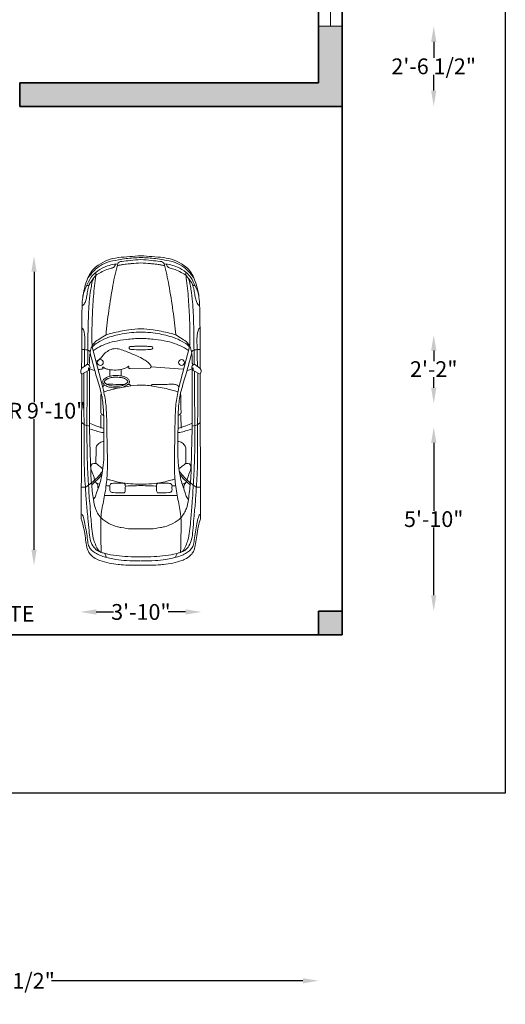
# Model space of a CAD drawing. Units: inches. Extents: x 1054 to 1577, y 4847 to 5610.
# Tile 2 of 5: x 1393 to 1577, y 4847 to 5221. Entities that reach past the tile are written whole.
import ezdxf

# ---------------------------------------------------------------- set-up
doc = ezdxf.new("R2010")
doc.units = ezdxf.units.IN
doc.header["$MEASUREMENT"] = 0
for name, color, linetype, lineweight in [('A-ANNO-DIMS', 2, 'Continuous', 18), ('A-ANNO-TEXT', 7, 'Continuous', 18), ('A-ANNO-TTLB', 7, 'Continuous', 25), ('A-GLAZ', 4, 'Continuous', 18), ('A-SITE-VEHI', 8, 'Continuous', 13), ('A-WALL', 7, 'Continuous', 35)]:
    doc.layers.add(name, color=color, linetype=linetype, lineweight=lineweight)
doc.layers.add('A-WALL-PATT', color=240, linetype='Continuous', lineweight=13, true_color=0xed1f24)
doc.styles.get("Standard").update_dxf_attribs({"font": 'arial.ttf'})
doc.dimstyles.get("Standard").update_dxf_attribs({"dimtxt": 6, "dimasz": 6, "dimexe": 0.18, "dimexo": 0.0625, "dimgap": 0.09, "dimtad": 0, "dimtih": 1, "dimtoh": 1, "dimdec": 1, "dimzin": 0, "dimdsep": 46, "dimlunit": 3, "dimtxsty": 'Standard', "dimcen": 0.09, "dimse1": 1, "dimse2": 1, "dimadec": 0, "dimazin": 0, "dimtfac": 1, "dimtdec": 1, "dimtofl": 0, "dimtmove": 0, "dimatfit": 3, "dimfxl": 1, "dimtolj": 1, "dimtzin": 0, "dimarcsym": 0})

# ---------------------------------------------------------------- blocks, each defined once
blk = doc.blocks.new('A$C242571DA')
for p, q in [((1660, 1632), (1714, 1733)), ((1714, 1733), (3817, 1740)), ((1317, 1580), (1910, 1425)), ((1638, 1619), (1625, 1632)), ((1625, 1632), (1660, 1632)), ((1638, 1619), (2503, 1619)), ((1660, 1548), (1638, 1619)), ((1682, 1652), (2695, 1655)), ((1700, 1699), (2985, 1696)), ((2503, 1619), (2862, 1608)), ((1644, 1489), (1610, 1020)), ((2312, 1454), (2501, 1457)), ((3007, 1527), (2808, 1525)), ((3475, 1401), (3475, 843)), ((4315, 1398), (4377, 1370)), ((1626, 1007), (1633, 720)), ((3475, 346), (3475, 904)), ((1740, 585), (1649, 587)), ((1317, 167), (1910, 322)), ((1746, 421), (1649, 421)), ((2312, 292), (2501, 290)), ((4315, 349), (4377, 376)), ((1660, 199), (1638, 128)), ((3007, 220), (2808, 222)), ((1638, 128), (1625, 115)), ((1625, 115), (1660, 115)), ((1638, 128), (2503, 128)), ((1660, 115), (1714, 14)), ((1682, 95), (2695, 91)), ((1700, 47), (2985, 51)), ((1714, 14), (3817, 7)), ((2503, 128), (2862, 139))]:
    blk.add_line(p, q)
for centre in [(1546, 1463), (1546, 284)]:
    blk.add_ellipse(centre, major_axis=(0, 42.9), ratio=0.983266, start_param=4.712389, end_param=10.995574)
for points, knots in [([(0, 873), (0, 928), (16, 1089), (26, 1310), (121, 1476), (189, 1569), (273, 1623), (370, 1666), (483, 1695), (561, 1715), (605, 1716)], [0, 0, 0, 0, 0.16039, 0.479033, 0.632967, 0.722015, 0.817474, 0.927562, 1.03733, 1.167094, 1.167094, 1.167094, 1.167094]), ([(605, 1716), (546, 1714), (449, 1665), (321, 1611), (225, 1521), (147, 1391), (122, 1275), (114, 1209)], [0, 0, 0, 0, 0.1772572, 0.3124951, 0.4151678, 0.5597243, 0.7575412, 0.7575412, 0.7575412, 0.7575412]), ([(723, 1727), (721, 1715), (694, 1690), (643, 1672), (574, 1655), (508, 1647), (455, 1635), (429, 1627), (417, 1624)], [0, 0, 0, 0, 0.034703, 0.0959761, 0.1659336, 0.2471559, 0.2929944, 0.3295918, 0.3295918, 0.3295918, 0.3295918]), ([(605, 1716), (642, 1723), (789, 1729), (1039, 1732), (1344, 1730), (1542, 1733), (1634, 1734)], [0, 0, 0, 0, 0.114897, 0.437061, 0.754269, 1.029686, 1.029686, 1.029686, 1.029686]), ([(1044, 1729), (1049, 1718), (1081, 1704), (1139, 1688), (1238, 1686), (1395, 1691), (1522, 1692), (1601, 1693)], [0, 0, 0, 0, 0.0364992, 0.0923739, 0.1867837, 0.3273982, 0.5667068, 0.5667068, 0.5667068, 0.5667068]), ([(1357, 1732), (1357, 1713), (1360, 1679), (1364, 1630), (1383, 1614), (1391, 1607)], [0, 0, 0, 0, 1.462159, 2.651105, 3.386321, 3.386321, 3.386321, 3.386321]), ([(1714, 1733), (1708, 1738), (1683, 1753), (1629, 1741), (1606, 1691), (1562, 1652), (1594, 1610), (1628, 1608), (1638, 1619)], [0, 0, 0, 0, 0.024864, 0.0846267, 0.1362471, 0.1900683, 0.2245199, 0.2681841, 0.2681841, 0.2681841, 0.2681841]), ([(2415, 1735), (2425, 1723), (2447, 1699), (2461, 1658), (2468, 1629), (2468, 1616)], [1.808086, 1.808086, 1.808086, 1.808086, 2.918874, 4.131288, 5.10151, 5.10151, 5.10151, 5.10151]), ([(3357, 1739), (3355, 1719), (3361, 1678), (3324, 1632), (3255, 1544), (3187, 1476), (3125, 1432)], [0, 0, 0, 0, 0.0597371, 0.1139981, 0.1672498, 0.3938869, 0.3938869, 0.3938869, 0.3938869]), ([(3745, 1737), (3749, 1730), (3764, 1717), (3811, 1699), (3895, 1687), (4003, 1663), (4108, 1649), (4196, 1638), (4259, 1603), (4302, 1550), (4340, 1484), (4365, 1408), (4390, 1324), (4398, 1267), (4402, 1235)], [0, 0, 0, 0, 0.0219205, 0.0572122, 0.1522539, 0.2718866, 0.3894011, 0.4710097, 0.5346344, 0.5986698, 0.6733118, 0.758696, 0.8351341, 0.9293726, 0.9293726, 0.9293726, 0.9293726]), ([(3817, 1740), (3833, 1730), (3883, 1718), (3973, 1695), (4085, 1680), (4194, 1663), (4281, 1644), (4344, 1598), (4390, 1540), (4427, 1449), (4458, 1337), (4476, 1233), (4478, 1175), (4479, 1162)], [0, 0, 0, 0, 0.056668, 0.14946, 0.28161, 0.392935, 0.481686, 0.542967, 0.622845, 0.69797, 0.833643, 0.965665, 1.00577, 1.00577, 1.00577, 1.00577]), ([(311, 1637), (282, 1614), (230, 1570), (149, 1486), (85, 1361), (60, 1219), (33, 1054), (25, 945), (25, 873)], [0, 0, 0, 0, 0.1095129, 0.2035347, 0.3452507, 0.5161382, 0.6275464, 0.8383798, 0.8383798, 0.8383798, 0.8383798]), ([(427, 1657), (429, 1647), (427, 1625), (400, 1617), (368, 1594), (328, 1565), (272, 1524), (237, 1452), (196, 1377), (184, 1315), (170, 1280), (157, 1254), (133, 1244), (119, 1243)], [0, 0, 0, 0, 0.0304541, 0.0502818, 0.0786089, 0.1479133, 0.1986294, 0.2831705, 0.3780326, 0.4523267, 0.4667809, 0.4902599, 0.5347198, 0.5347198, 0.5347198, 0.5347198]), ([(1317, 1580), (1228, 1586), (1036, 1585), (741, 1573), (486, 1553), (333, 1534), (283, 1528)], [0, 0, 0, 0, 0.269375, 0.574535, 0.885339, 1.036319, 1.036319, 1.036319, 1.036319]), ([(324, 1558), (345, 1572), (400, 1585), (516, 1607), (680, 1626), (885, 1636), (1117, 1642), (1346, 1644), (1505, 1645), (1574, 1646)], [0, 0, 0, 0, 0.076148, 0.165903, 0.355672, 0.569871, 0.782325, 1.050047, 1.257936, 1.257936, 1.257936, 1.257936]), ([(1555, 1618), (1528, 1618), (1473, 1620), (1393, 1609), (1318, 1591), (1249, 1545), (1201, 1467), (1143, 1386), (1105, 1240), (1076, 1072), (1056, 932), (1056, 873)], [0, 0, 0, 0, 0.082256, 0.165174, 0.241383, 0.30939, 0.405348, 0.511507, 0.603349, 0.843635, 1.017671, 1.017671, 1.017671, 1.017671]), ([(1317, 1580), (1297, 1556), (1248, 1494), (1178, 1350), (1124, 1137), (1106, 965), (1106, 873)], [0, 0, 0, 0, 0.0947759, 0.2311242, 0.4700259, 0.7400315, 0.7400315, 0.7400315, 0.7400315]), ([(3536, 1563), (3520, 1551), (3484, 1526), (3408, 1511), (3323, 1473), (3208, 1445), (3073, 1422), (2867, 1405), (2626, 1413), (2397, 1411), (2201, 1417), (2001, 1438), (1732, 1526), (1528, 1579), (1408, 1611)], [0, 0, 0, 0, 0.05975, 0.126928, 0.230034, 0.336675, 0.482225, 0.641324, 0.954906, 1.203173, 1.330375, 1.542773, 1.802261, 2.175545, 2.175545, 2.175545, 2.175545]), ([(1574, 1646), (1573, 1638), (1574, 1622), (1560, 1619), (1555, 1618)], [0, 0, 0, 0, 0.02274132, 0.03717479, 0.03717479, 0.03717479, 0.03717479]), ([(2424, 1619), (2442, 1590), (2464, 1519), (2495, 1451), (2502, 1411)], [0, 0, 0, 0, 0.1000351, 0.2184418, 0.2184418, 0.2184418, 0.2184418]), ([(2508, 1618), (2521, 1588), (2537, 1527), (2560, 1458), (2563, 1421), (2564, 1411)], [0, 0, 0, 0, 2.528586, 4.711885, 5.408215, 5.408215, 5.408215, 5.408215]), ([(2695, 1655), (2830, 1655), (3041, 1651), (3351, 1631), (3527, 1623), (3627, 1612)], [0, 0, 0, 0, 0.4042759, 0.6333827, 0.9326252, 0.9326252, 0.9326252, 0.9326252]), ([(2862, 1608), (2921, 1607), (3047, 1601), (3191, 1602), (3357, 1584), (3498, 1571), (3623, 1549), (3664, 1533)], [0, 0, 0, 0, 0.1783018, 0.3787173, 0.431954, 0.6762374, 0.8077184, 0.8077184, 0.8077184, 0.8077184]), ([(2985, 1696), (3051, 1696), (3172, 1691), (3367, 1678), (3575, 1664), (3788, 1644), (3968, 1628), (4104, 1617), (4204, 1578), (4272, 1519), (4301, 1452), (4342, 1305), (4362, 1111), (4367, 937), (4367, 873)], [0, 0, 0, 0, 0.198873, 0.363323, 0.587433, 0.823543, 1.004622, 1.129816, 1.230113, 1.320655, 1.388577, 1.443334, 1.771447, 1.958652, 1.958652, 1.958652, 1.958652]), ([(3248, 1545), (3227, 1550), (3176, 1562), (3114, 1593), (3053, 1605), (3010, 1579), (3010, 1545), (3010, 1516), (3034, 1500), (3053, 1465), (3079, 1444), (3084, 1424)], [0, 0, 0, 0, 0.0655106, 0.1550445, 0.2094604, 0.2438604, 0.287164, 0.3001388, 0.3275984, 0.3616951, 0.4200969, 0.4200969, 0.4200969, 0.4200969]), ([(3319, 1587), (3303, 1568), (3257, 1517), (3207, 1467), (3171, 1440)], [0, 0, 0, 0, 1.868162, 5.271297, 5.271297, 5.271297, 5.271297]), ([(3627, 1612), (3702, 1609), (3826, 1597), (3991, 1583), (4112, 1562), (4212, 1523), (4290, 1488), (4301, 1448)], [0, 0, 0, 0, 0.2277977, 0.3719478, 0.4996814, 0.5863441, 0.709615, 0.709615, 0.709615, 0.709615]), ([(1373, 1563), (1357, 1545), (1322, 1490), (1277, 1386), (1233, 1244), (1211, 1069), (1197, 942), (1197, 873)], [0, 0, 0, 0, 0.0708922, 0.1925846, 0.3348457, 0.5072814, 0.7109928, 0.7109928, 0.7109928, 0.7109928]), ([(1910, 1425), (1933, 1419), (1996, 1408), (2094, 1386), (2212, 1377), (2419, 1367), (2705, 1366), (3033, 1354), (3316, 1371), (3559, 1416), (3789, 1462), (4029, 1453), (4196, 1455), (4293, 1448), (4301, 1448)], [0, 0, 0, 0, 0.073325, 0.188896, 0.303039, 0.425821, 0.811242, 1.159737, 1.41058, 1.660623, 1.899627, 2.11145, 2.377727, 2.401703, 2.401703, 2.401703, 2.401703]), ([(1997, 1450), (2040, 1455), (2127, 1452), (2220, 1454), (2287, 1457), (2306, 1434), (2313, 1420), (2316, 1414)], [0, 0, 0, 0, 3.267856, 6.568708, 7.399663, 8.099385, 8.621705, 8.621705, 8.621705, 8.621705]), ([(2808, 1525), (2792, 1525), (2752, 1520), (2711, 1473), (2690, 1431), (2691, 1410)], [0, 0, 0, 0, 0.0486628, 0.1144515, 0.1777721, 0.1777721, 0.1777721, 0.1777721]), ([(3275, 1533), (3288, 1528), (3300, 1505), (3308, 1482), (3312, 1473)], [0, 0, 0, 0, 0.983949, 1.771691, 1.771691, 1.771691, 1.771691]), ([(3372, 1495), (3354, 1497), (3316, 1495), (3292, 1526), (3275, 1533)], [0, 0, 0, 0, 0.0535488, 0.1060573, 0.1060573, 0.1060573, 0.1060573]), ([(3664, 1533), (3687, 1526), (3735, 1502), (3817, 1445), (3884, 1343), (3925, 1240), (3937, 1177), (3940, 1158)], [0, 0, 0, 0, 0.0720749, 0.1581284, 0.2958089, 0.4262456, 0.4842292, 0.4842292, 0.4842292, 0.4842292]), ([(114, 1209), (215, 1239), (443, 1285), (788, 1339), (1030, 1371), (1146, 1379)], [0, 0, 0, 0, 0.317374, 0.69576, 1.04714, 1.04714, 1.04714, 1.04714]), ([(1898, 1426), (1889, 1421), (1871, 1397), (1856, 1345), (1868, 1234), (1864, 1132), (1863, 1038), (1877, 1022), (1885, 1016)], [0, 0, 0, 0, 0.842998, 2.122875, 3.997599, 9.174838, 10.012722, 10.751336, 10.751336, 10.751336, 10.751336]), ([(1970, 1407), (1960, 1370), (1927, 1259), (1891, 1078), (1874, 933), (1874, 864)], [0, 0, 0, 0, 0.1139079, 0.3411539, 0.543502, 0.543502, 0.543502, 0.543502]), ([(3232, 1368), (3241, 1356), (3253, 1316), (3272, 1241), (3298, 1128), (3311, 975), (3311, 858), (3312, 794)], [0, 0, 0, 0, 0.0451009, 0.1211996, 0.2308505, 0.385263, 0.5739042, 0.5739042, 0.5739042, 0.5739042]), ([(3295, 1175), (3295, 1207), (3300, 1250), (3298, 1304), (3326, 1329), (3364, 1321), (3399, 1329), (3422, 1316), (3431, 1298), (3439, 1234), (3440, 1174), (3435, 1112), (3419, 1102), (3396, 1099), (3363, 1101), (3331, 1097), (3299, 1108), (3297, 1140), (3295, 1161), (3295, 1175)], [0, 0, 0, 0, 0.0969044, 0.1295913, 0.1506192, 0.1985921, 0.2360698, 0.2557908, 0.2719711, 0.2929882, 0.44406, 0.4519132, 0.4720918, 0.4918599, 0.5228758, 0.5707096, 0.5892096, 0.6145759, 0.654681, 0.654681, 0.654681, 0.654681]), ([(114, 1209), (103, 1207), (84, 1188), (76, 1122), (68, 1017), (53, 925), (53, 873)], [0, 0, 0, 0, 0.0314754, 0.0702057, 0.1915753, 0.3439346, 0.3439346, 0.3439346, 0.3439346]), ([(136, 1213), (139, 1212), (138, 1193), (133, 1168), (119, 1112), (116, 1059), (109, 975), (102, 920), (102, 873)], [0, 0, 0, 0, 0.0114788, 0.0403472, 0.0875838, 0.1755608, 0.1991501, 0.3369659, 0.3369659, 0.3369659, 0.3369659]), ([(3940, 1158), (3950, 1111), (3964, 1016), (3960, 921), (3960, 873)], [0, 0, 0, 0, 0.140379, 0.2808468, 0.2808468, 0.2808468, 0.2808468]), ([(4402, 1235), (4412, 1185), (4422, 1066), (4424, 946), (4424, 878)], [0, 0, 0, 0, 0.1502861, 0.3522699, 0.3522699, 0.3522699, 0.3522699]), ([(1311, 873), (1311, 902), (1309, 951), (1315, 1002), (1314, 1039), (1332, 1045), (1346, 1044), (1357, 1029), (1359, 970), (1362, 918), (1363, 873)], [0, 0, 0, 0, 0.0857277, 0.1381048, 0.1641986, 0.1769751, 0.1890325, 0.2028129, 0.2286049, 0.3592554, 0.3592554, 0.3592554, 0.3592554]), ([(1626, 1007), (1623, 1013), (1603, 1029), (1559, 995), (1523, 952), (1480, 878), (1431, 774), (1385, 658), (1344, 551), (1343, 462), (1380, 387), (1428, 330), (1480, 295), (1510, 257), (1525, 233), (1528, 222)], [0, 0, 0, 0, 0.527288, 1.647451, 3.487558, 5.099073, 7.968657, 12.238313, 14.475187, 16.613757, 18.744202, 20.639343, 22.223389, 23.452731, 24.286529, 24.286529, 24.286529, 24.286529]), ([(3339, 1099), (3339, 1095), (3336, 1011), (3333, 926), (3330, 846)], [11.235438, 11.235438, 11.235438, 11.235438, 11.552536, 17.586883, 17.586883, 17.586883, 17.586883]), ([(0, 873), (0, 819), (16, 658), (26, 437), (121, 270), (189, 178), (273, 124), (370, 80), (483, 52), (561, 32), (605, 31)], [0, 0, 0, 0, 0.16039, 0.479033, 0.632967, 0.722015, 0.817474, 0.927562, 1.03733, 1.167094, 1.167094, 1.167094, 1.167094]), ([(311, 109), (282, 133), (230, 177), (149, 261), (85, 385), (60, 528), (33, 692), (25, 802), (25, 873)], [0, 0, 0, 0, 0.1095129, 0.2035347, 0.3452507, 0.5161382, 0.6275464, 0.8383798, 0.8383798, 0.8383798, 0.8383798]), ([(114, 538), (103, 540), (84, 559), (76, 625), (68, 729), (53, 822), (53, 873)], [0, 0, 0, 0, 0.0314754, 0.0702057, 0.1915753, 0.3439346, 0.3439346, 0.3439346, 0.3439346]), ([(136, 534), (139, 535), (138, 553), (133, 578), (119, 635), (116, 688), (109, 772), (102, 827), (102, 873)], [0, 0, 0, 0, 0.0114788, 0.0403472, 0.0875838, 0.1755608, 0.1991501, 0.3369659, 0.3369659, 0.3369659, 0.3369659]), ([(1555, 129), (1528, 129), (1473, 126), (1393, 138), (1318, 156), (1249, 201), (1201, 280), (1143, 361), (1105, 506), (1076, 674), (1056, 814), (1056, 873)], [0, 0, 0, 0, 0.082256, 0.165174, 0.241383, 0.30939, 0.405348, 0.511507, 0.603349, 0.843635, 1.017671, 1.017671, 1.017671, 1.017671]), ([(1317, 167), (1297, 191), (1248, 252), (1178, 396), (1124, 609), (1106, 782), (1106, 873)], [0, 0, 0, 0, 0.0947759, 0.2311242, 0.4700259, 0.7400315, 0.7400315, 0.7400315, 0.7400315]), ([(1373, 184), (1357, 202), (1322, 257), (1277, 361), (1233, 503), (1211, 677), (1197, 804), (1197, 873)], [0, 0, 0, 0, 0.0708922, 0.1925846, 0.3348457, 0.5072814, 0.7109928, 0.7109928, 0.7109928, 0.7109928]), ([(1311, 873), (1311, 844), (1309, 796), (1315, 745), (1314, 707), (1332, 702), (1346, 703), (1357, 718), (1359, 777), (1362, 829), (1363, 873)], [0, 0, 0, 0, 0.0857277, 0.1381048, 0.1641986, 0.1769751, 0.1890325, 0.2028129, 0.2286049, 0.3592554, 0.3592554, 0.3592554, 0.3592554]), ([(1970, 339), (1960, 377), (1927, 488), (1893, 663), (1874, 802), (1874, 864)], [0, 0, 0, 0, 0.1139079, 0.3411539, 0.5260188, 0.5260188, 0.5260188, 0.5260188]), ([(2985, 51), (3051, 51), (3172, 56), (3367, 69), (3575, 82), (3788, 103), (3968, 119), (4104, 130), (4204, 169), (4272, 227), (4301, 295), (4342, 441), (4362, 636), (4367, 810), (4367, 873)], [0, 0, 0, 0, 0.198873, 0.363323, 0.587433, 0.823543, 1.004622, 1.129816, 1.230113, 1.320655, 1.388577, 1.443334, 1.771447, 1.958652, 1.958652, 1.958652, 1.958652]), ([(3232, 379), (3241, 391), (3253, 431), (3272, 506), (3298, 619), (3311, 772), (3311, 888), (3312, 952)], [0, 0, 0, 0, 0.0451009, 0.1211996, 0.2308505, 0.385263, 0.5739042, 0.5739042, 0.5739042, 0.5739042]), ([(3339, 648), (3339, 652), (3336, 736), (3333, 820), (3330, 901)], [11.235438, 11.235438, 11.235438, 11.235438, 11.552536, 17.586883, 17.586883, 17.586883, 17.586883]), ([(3940, 589), (3950, 636), (3964, 730), (3960, 826), (3960, 873)], [0, 0, 0, 0, 0.140379, 0.2808468, 0.2808468, 0.2808468, 0.2808468]), ([(4402, 512), (4412, 561), (4422, 681), (4424, 800), (4424, 869)], [0, 0, 0, 0, 0.1502861, 0.3522699, 0.3522699, 0.3522699, 0.3522699]), ([(1639, 326), (1635, 324), (1629, 318), (1613, 315), (1612, 324), (1613, 330), (1619, 338), (1629, 346), (1638, 366), (1649, 405), (1656, 473), (1656, 543), (1645, 611), (1623, 651), (1615, 684), (1598, 691), (1604, 697), (1610, 700), (1619, 699), (1626, 701), (1638, 699), (1633, 713), (1633, 720)], [0, 0, 0, 0, 0.0138597, 0.0278304, 0.0329137, 0.0379971, 0.0465756, 0.0592704, 0.0762214, 0.1105991, 0.1789801, 0.2766959, 0.3173629, 0.3800771, 0.4110544, 0.4160421, 0.4210284, 0.4277212, 0.4387433, 0.4448131, 0.4508005, 0.4694463, 0.4694463, 0.4694463, 0.4694463]), ([(1863, 686), (1864, 694), (1865, 711), (1877, 724), (1885, 731)], [9.436432, 9.436432, 9.436432, 9.436432, 10.012722, 10.751336, 10.751336, 10.751336, 10.751336]), ([(1740, 585), (1738, 572), (1750, 644), (1766, 664), (1792, 700), (1821, 710), (1853, 704), (1874, 668), (1905, 623), (1916, 557), (1915, 484), (1906, 418), (1885, 363), (1859, 329), (1831, 318), (1811, 323), (1792, 329), (1778, 350), (1753, 386), (1738, 466), (1729, 497), (1742, 598), (1740, 585)], [0, 0, 0, 0, 0.03969, 0.089634, 0.13125, 0.1542862, 0.1797268, 0.2207266, 0.2680991, 0.3447665, 0.4095645, 0.4843001, 0.541515, 0.5817687, 0.6060665, 0.6262474, 0.6436722, 0.6634686, 0.6988791, 0.7758465, 0.8696394, 0.907731, 0.907731, 0.907731, 0.907731]), ([(1765, 587), (1766, 591), (1766, 595), (1769, 606), (1770, 611), (1773, 627), (1776, 633), (1780, 642), (1782, 645), (1786, 651), (1787, 653), (1793, 660), (1797, 666), (1804, 674), (1807, 676), (1811, 679), (1813, 680), (1817, 682), (1819, 683), (1824, 683), (1828, 683), (1832, 682), (1834, 682), (1836, 680), (1838, 679), (1842, 674), (1845, 670), (1850, 662), (1853, 657), (1859, 647), (1862, 643), (1868, 633), (1871, 627), (1877, 616), (1879, 610), (1883, 597), (1884, 591), (1888, 571), (1890, 556), (1891, 527), (1891, 513), (1889, 470), (1885, 441), (1874, 404), (1871, 394), (1863, 379), (1861, 373), (1854, 364), (1851, 359), (1845, 353), (1842, 350), (1836, 346), (1833, 345), (1829, 345), (1828, 345), (1825, 345), (1823, 345), (1818, 346), (1815, 347), (1811, 349), (1809, 349), (1808, 350), (1808, 350), (1807, 351), (1807, 352), (1805, 354), (1803, 356), (1800, 361), (1798, 364), (1795, 368), (1793, 370), (1789, 377), (1787, 381), (1782, 389), (1780, 394), (1777, 403), (1775, 408), (1771, 423), (1768, 434), (1765, 450), (1764, 456), (1761, 467), (1760, 471), (1758, 484), (1757, 493), (1758, 511), (1758, 516), (1759, 528), (1759, 534), (1761, 554), (1763, 571), (1764, 581), (1765, 583), (1765, 585), (1765, 585), (1765, 586), (1765, 587), (1765, 587)], [0.497033, 0.497033, 0.497033, 0.497033, 0.723444, 0.723444, 0.974636, 0.974636, 1.50964, 1.50964, 2.044645, 2.044645, 2.271061, 2.271061, 2.862376, 2.862376, 3.217654, 3.217654, 3.537253, 3.537253, 3.856852, 3.856852, 4.368613, 4.368613, 4.584627, 4.584627, 4.99269, 4.99269, 5.400753, 5.400753, 5.808816, 5.808816, 6.216879, 6.216879, 6.778716, 6.778716, 7.350371, 7.350371, 7.922025, 7.922025, 9.065335, 9.065335, 10.208644, 10.208644, 12.495263, 12.495263, 13.409896, 13.409896, 13.929088, 13.929088, 14.44828, 14.44828, 14.909885, 14.909885, 15.371489, 15.371489, 15.62524, 15.62524, 15.87899, 15.87899, 16.120875, 16.120875, 16.36276, 16.36276, 16.51635, 16.51635, 16.669941, 16.669941, 16.921521, 16.921521, 17.136676, 17.136676, 17.351831, 17.351831, 17.782142, 17.782142, 18.204974, 18.204974, 18.627807, 18.627807, 19.473473, 19.473473, 19.978923, 19.978923, 20.484372, 20.484372, 21.475119, 21.475119, 21.859144, 21.859144, 22.162884, 22.162884, 22.770362, 22.770362, 22.900493, 22.900493, 22.951221, 22.951221, 22.964298, 22.964298, 22.964298, 22.964298]), ([(1864, 379), (1863, 384), (1858, 414), (1867, 502), (1865, 581), (1864, 639)], [1.749253, 1.749253, 1.749253, 1.749253, 2.122875, 3.997599, 8.307432, 8.307432, 8.307432, 8.307432]), ([(3295, 572), (3295, 539), (3300, 497), (3298, 443), (3326, 418), (3364, 426), (3399, 417), (3422, 431), (3431, 449), (3439, 513), (3440, 572), (3435, 635), (3419, 645), (3396, 648), (3363, 646), (3331, 650), (3299, 639), (3297, 606), (3295, 586), (3295, 572)], [0, 0, 0, 0, 0.0969044, 0.1295913, 0.1506192, 0.1985921, 0.2360698, 0.2557908, 0.2719711, 0.2929882, 0.44406, 0.4519132, 0.4720918, 0.4918599, 0.5228758, 0.5707096, 0.5892096, 0.6145759, 0.654681, 0.654681, 0.654681, 0.654681]), ([(3664, 214), (3687, 221), (3735, 244), (3817, 302), (3884, 404), (3925, 507), (3937, 570), (3940, 589)], [0, 0, 0, 0, 0.0720749, 0.1581284, 0.2958089, 0.4262456, 0.4842292, 0.4842292, 0.4842292, 0.4842292]), ([(3817, 7), (3833, 17), (3883, 29), (3973, 52), (4085, 66), (4194, 84), (4281, 102), (4344, 149), (4390, 206), (4427, 298), (4458, 410), (4476, 513), (4478, 572), (4479, 585)], [0, 0, 0, 0, 0.056668, 0.14946, 0.28161, 0.392935, 0.481686, 0.542967, 0.622845, 0.69797, 0.833643, 0.965665, 1.00577, 1.00577, 1.00577, 1.00577]), ([(605, 31), (546, 32), (449, 82), (321, 136), (225, 226), (147, 356), (122, 472), (114, 538)], [0, 0, 0, 0, 0.1772572, 0.3124951, 0.4151678, 0.5597243, 0.7575412, 0.7575412, 0.7575412, 0.7575412]), ([(114, 538), (215, 508), (443, 462), (788, 408), (1030, 376), (1146, 368)], [0, 0, 0, 0, 0.317374, 0.69576, 1.04714, 1.04714, 1.04714, 1.04714]), ([(427, 90), (429, 100), (427, 122), (400, 130), (368, 153), (328, 182), (272, 223), (237, 295), (196, 370), (184, 432), (170, 467), (157, 493), (133, 502), (119, 504)], [0, 0, 0, 0, 0.0304541, 0.0502818, 0.0786089, 0.1479133, 0.1986294, 0.2831705, 0.3780326, 0.4523267, 0.4667809, 0.4902599, 0.5347198, 0.5347198, 0.5347198, 0.5347198]), ([(3745, 10), (3749, 17), (3764, 30), (3811, 48), (3895, 60), (4003, 84), (4108, 98), (4196, 108), (4259, 144), (4302, 197), (4340, 263), (4365, 339), (4390, 422), (4398, 480), (4402, 512)], [0, 0, 0, 0, 0.0219205, 0.0572122, 0.1522539, 0.2718866, 0.3894011, 0.4710097, 0.5346344, 0.5986698, 0.6733118, 0.758696, 0.8351341, 0.9293726, 0.9293726, 0.9293726, 0.9293726]), ([(3536, 184), (3520, 196), (3484, 221), (3408, 236), (3323, 274), (3208, 302), (3073, 325), (2867, 342), (2626, 334), (2397, 336), (2201, 330), (2001, 309), (1732, 221), (1528, 168), (1408, 136)], [0, 0, 0, 0, 0.05975, 0.126928, 0.230034, 0.336675, 0.482225, 0.641324, 0.954906, 1.203173, 1.330375, 1.542773, 1.802261, 2.175545, 2.175545, 2.175545, 2.175545]), ([(1898, 321), (1889, 326), (1881, 337), (1875, 348), (1874, 350)], [0, 0, 0, 0, 0.8429982, 0.9626806, 0.9626806, 0.9626806, 0.9626806]), ([(1910, 322), (1933, 328), (1996, 339), (2094, 361), (2212, 370), (2419, 380), (2705, 380), (3033, 393), (3316, 376), (3559, 331), (3789, 285), (4029, 294), (4196, 292), (4293, 299), (4301, 299)], [0, 0, 0, 0, 0.073325, 0.188896, 0.303039, 0.425821, 0.811242, 1.159737, 1.41058, 1.660623, 1.899627, 2.11145, 2.377727, 2.401703, 2.401703, 2.401703, 2.401703]), ([(1997, 296), (2040, 292), (2127, 295), (2220, 292), (2287, 290), (2306, 312), (2313, 327), (2316, 333)], [0, 0, 0, 0, 3.267856, 6.568708, 7.399663, 8.099385, 8.621705, 8.621705, 8.621705, 8.621705]), ([(2424, 128), (2442, 157), (2464, 228), (2495, 296), (2502, 335)], [0, 0, 0, 0, 0.1000351, 0.2184418, 0.2184418, 0.2184418, 0.2184418]), ([(2508, 128), (2521, 159), (2537, 220), (2560, 288), (2563, 326), (2564, 335)], [0, 0, 0, 0, 2.528586, 4.711885, 5.408215, 5.408215, 5.408215, 5.408215]), ([(2808, 222), (2792, 222), (2752, 227), (2711, 274), (2690, 316), (2691, 337)], [0, 0, 0, 0, 0.0486628, 0.1144515, 0.1777721, 0.1777721, 0.1777721, 0.1777721]), ([(3248, 202), (3227, 196), (3176, 185), (3114, 154), (3053, 141), (3010, 168), (3010, 201), (3010, 231), (3034, 247), (3053, 282), (3079, 303), (3084, 322)], [0, 0, 0, 0, 0.0655106, 0.1550445, 0.2094604, 0.2438604, 0.287164, 0.3001388, 0.3275984, 0.3616951, 0.4200969, 0.4200969, 0.4200969, 0.4200969]), ([(3357, 7), (3355, 28), (3361, 69), (3324, 115), (3255, 203), (3187, 271), (3125, 315)], [0, 0, 0, 0, 0.0597371, 0.1139981, 0.1672498, 0.3938869, 0.3938869, 0.3938869, 0.3938869]), ([(3319, 160), (3303, 179), (3257, 230), (3207, 280), (3171, 307)], [0, 0, 0, 0, 1.868162, 5.271297, 5.271297, 5.271297, 5.271297]), ([(3627, 135), (3702, 138), (3826, 150), (3991, 164), (4112, 184), (4212, 224), (4290, 259), (4301, 299)], [0, 0, 0, 0, 0.2277977, 0.3719478, 0.4996814, 0.5863441, 0.709615, 0.709615, 0.709615, 0.709615]), ([(1317, 167), (1228, 161), (1036, 162), (741, 174), (486, 193), (333, 212), (283, 218)], [0, 0, 0, 0, 0.269375, 0.574535, 0.885339, 1.036319, 1.036319, 1.036319, 1.036319]), ([(324, 189), (345, 175), (400, 162), (516, 140), (680, 121), (885, 111), (1117, 105), (1346, 103), (1505, 102), (1574, 101)], [0, 0, 0, 0, 0.076148, 0.165903, 0.355672, 0.569871, 0.782325, 1.050047, 1.257936, 1.257936, 1.257936, 1.257936]), ([(2862, 139), (2921, 139), (3047, 146), (3191, 145), (3357, 163), (3498, 176), (3623, 197), (3664, 214)], [0, 0, 0, 0, 0.1783018, 0.3787173, 0.431954, 0.6762374, 0.8077184, 0.8077184, 0.8077184, 0.8077184]), ([(3275, 214), (3288, 218), (3300, 242), (3308, 264), (3312, 274)], [0, 0, 0, 0, 0.983949, 1.771691, 1.771691, 1.771691, 1.771691]), ([(3372, 251), (3354, 250), (3316, 252), (3292, 221), (3275, 214)], [0, 0, 0, 0, 0.0535488, 0.1060573, 0.1060573, 0.1060573, 0.1060573]), ([(723, 20), (721, 32), (694, 57), (643, 75), (574, 91), (508, 100), (455, 112), (429, 119), (417, 123)], [0, 0, 0, 0, 0.034703, 0.0959761, 0.1659336, 0.2471559, 0.2929944, 0.3295918, 0.3295918, 0.3295918, 0.3295918]), ([(605, 31), (642, 23), (789, 18), (1039, 15), (1344, 17), (1542, 14), (1634, 13)], [0, 0, 0, 0, 0.114897, 0.437061, 0.754269, 1.029686, 1.029686, 1.029686, 1.029686]), ([(1044, 18), (1049, 29), (1081, 43), (1139, 59), (1238, 61), (1395, 55), (1522, 54), (1601, 54)], [0, 0, 0, 0, 0.0364992, 0.0923739, 0.1867837, 0.3273982, 0.5667068, 0.5667068, 0.5667068, 0.5667068]), ([(1357, 15), (1357, 34), (1360, 68), (1364, 116), (1383, 133), (1391, 140)], [0, 0, 0, 0, 1.462159, 2.651105, 3.386321, 3.386321, 3.386321, 3.386321]), ([(1574, 101), (1573, 109), (1574, 125), (1560, 128), (1555, 129)], [0, 0, 0, 0, 0.02274132, 0.03717479, 0.03717479, 0.03717479, 0.03717479]), ([(1714, 14), (1708, 9), (1683, -6), (1629, 6), (1606, 55), (1562, 94), (1594, 137), (1628, 138), (1638, 128)], [0, 0, 0, 0, 0.024864, 0.0846267, 0.1362471, 0.1900683, 0.2245199, 0.2681841, 0.2681841, 0.2681841, 0.2681841]), ([(2415, 12), (2425, 24), (2447, 48), (2461, 89), (2468, 118), (2468, 131)], [1.808086, 1.808086, 1.808086, 1.808086, 2.918874, 4.131288, 5.10151, 5.10151, 5.10151, 5.10151]), ([(2695, 91), (2830, 92), (3041, 95), (3351, 116), (3527, 124), (3627, 135)], [0, 0, 0, 0, 0.4042759, 0.6333827, 0.9326252, 0.9326252, 0.9326252, 0.9326252])]:
    blk.add_open_spline(points, degree=3, knots=knots)
for points in [[(283, 1528), (268, 1525), (251, 1528), (235, 1528)], [(3332, 1378), (3334, 1360), (3336, 1342), (3337, 1325)], [(4479, 1162), (4491, 1066), (4488, 969), (4488, 873)], [(4479, 585), (4491, 681), (4488, 777), (4488, 873)], [(1646, 253), (1648, 277), (1640, 302), (1639, 326)], [(3332, 369), (3334, 386), (3336, 404), (3337, 422)], [(283, 218), (268, 222), (251, 219), (235, 218)]]:
    blk.add_open_spline(points, degree=3)
blk = doc.blocks.new('WINDOW-36IN')
for p, q in [((0, 9), (0, 0)), ((36, 9), (0, 9)), ((36, 0), (36, 9)), ((36, 4.5), (0, 4.5)), ((0, 0), (36, 0))]:
    blk.add_line(p, q)
blk = doc.blocks.new('*D22')
at = {"layer": 'A-ANNO-DIMS', "color": 0, "lineweight": -2, "transparency": 16777216}
for p, q in [((1397.97, 5125.61), (1397.97, 5075.91)), ((1397.97, 5019.83), (1397.97, 5069.53))]:
    blk.add_line(p, q, dxfattribs=at)
at = {"layer": 'A-ANNO-DIMS', "color": 0, "transparency": 16777216}
for points in [[(1396.97, 5125.61), (1398.97, 5125.61), (1397.97, 5131.61)], [(1396.97, 5019.83), (1398.97, 5019.83), (1397.97, 5013.83)]]:
    blk.add_solid(points, dxfattribs=at)
at = {"layer": 'Defpoints', "color": 0, "transparency": 16777216}
for p in [(1415.63, 5131.61), (1397.97, 5013.83), (1415.63, 5013.83)]:
    blk.add_point(p, dxfattribs=at)
at = {"layer": 'A-ANNO-DIMS', "color": 0, "transparency": 16777216, "insert": (1397.97, 5072.72), "char_height": 6, "attachment_point": 5}
blk.add_mtext('\\A1;CAR 9\'-10"', dxfattribs=at)
blk = doc.blocks.new('*D23')
at = {"layer": 'A-ANNO-DIMS', "color": 0, "lineweight": -2, "transparency": 16777216}
for p, q in [((1421.63, 4996.16), (1428.25, 4996.16)), ((1455.66, 4996.16), (1449.04, 4996.16))]:
    blk.add_line(p, q, dxfattribs=at)
at = {"layer": 'A-ANNO-DIMS', "color": 0, "transparency": 16777216}
for points in [[(1421.63, 4997.16), (1421.63, 4995.16), (1415.63, 4996.16)], [(1455.66, 4997.16), (1455.66, 4995.16), (1461.66, 4996.16)]]:
    blk.add_solid(points, dxfattribs=at)
at = {"layer": 'Defpoints', "color": 0, "transparency": 16777216}
for p in [(1415.63, 5013.83), (1461.66, 5013.83), (1461.66, 4996.16)]:
    blk.add_point(p, dxfattribs=at)
at = {"layer": 'A-ANNO-DIMS', "color": 0, "transparency": 16777216, "insert": (1438.65, 4996.16), "char_height": 6, "attachment_point": 5}
blk.add_mtext('\\A1;3\'-10"', dxfattribs=at)
blk = doc.blocks.new('*D27')
at = {"layer": 'A-ANNO-DIMS', "color": 0, "lineweight": -2, "transparency": 16777216}
for p, q in [((1550.07, 5060.48), (1550.07, 5034.64)), ((1550.07, 5002.48), (1550.07, 5028.33))]:
    blk.add_line(p, q, dxfattribs=at)
at = {"layer": 'A-ANNO-DIMS', "color": 0, "transparency": 16777216}
for points in [[(1549.07, 5060.48), (1551.07, 5060.48), (1550.07, 5066.48)], [(1549.07, 5002.48), (1551.07, 5002.48), (1550.07, 4996.48)]]:
    blk.add_solid(points, dxfattribs=at)
at = {"layer": 'Defpoints', "color": 0, "transparency": 16777216}
for p in [(1139.77, 5066.48), (1550.07, 5066.48), (1139.77, 4996.48)]:
    blk.add_point(p, dxfattribs=at)
at = {"layer": 'A-ANNO-DIMS', "color": 0, "transparency": 16777216, "insert": (1550.07, 5031.48), "char_height": 6, "attachment_point": 5}
blk.add_mtext('\\A1;5\'-10"', dxfattribs=at)
blk = doc.blocks.new('*D28')
at = {"layer": 'A-ANNO-DIMS', "color": 0, "lineweight": -2, "transparency": 16777216}
for p, q in [((1274.77, 4855.83), (1370.42, 4855.83)), ((1500.27, 4855.83), (1404.63, 4855.83))]:
    blk.add_line(p, q, dxfattribs=at)
at = {"layer": 'A-ANNO-DIMS', "color": 0, "transparency": 16777216}
for points in [[(1274.77, 4856.83), (1274.77, 4854.83), (1268.77, 4855.83)], [(1500.27, 4856.83), (1500.27, 4854.83), (1506.27, 4855.83)]]:
    blk.add_solid(points, dxfattribs=at)
at = {"layer": 'Defpoints', "color": 0, "transparency": 16777216}
for p in [(1268.77, 4987.48), (1506.27, 4987.48), (1506.27, 4855.83)]:
    blk.add_point(p, dxfattribs=at)
at = {"layer": 'A-ANNO-DIMS', "color": 0, "transparency": 16777216, "insert": (1387.52, 4855.83), "char_height": 6, "attachment_point": 5}
blk.add_mtext('\\A1;19\'-9 1/2"', dxfattribs=at)
blk = doc.blocks.new('*D37')
at = {"layer": 'A-ANNO-DIMS', "color": 0, "lineweight": -2, "transparency": 16777216}
for p, q in [((1550.07, 5213.01), (1550.07, 5206.94)), ((1550.07, 5194.48), (1550.07, 5200.55))]:
    blk.add_line(p, q, dxfattribs=at)
at = {"layer": 'A-ANNO-DIMS', "color": 0, "transparency": 16777216}
for points in [[(1549.07, 5213.01), (1551.07, 5213.01), (1550.07, 5219.01)], [(1549.07, 5194.48), (1551.07, 5194.48), (1550.07, 5188.48)]]:
    blk.add_solid(points, dxfattribs=at)
at = {"layer": 'Defpoints', "color": 0, "transparency": 16777216}
for p in [(1515.27, 5219.01), (1550.07, 5219.01), (1515.27, 5188.48)]:
    blk.add_point(p, dxfattribs=at)
at = {"layer": 'A-ANNO-DIMS', "color": 0, "transparency": 16777216, "insert": (1550.07, 5203.74), "char_height": 6, "attachment_point": 5}
blk.add_mtext('\\A1;2\'-6 1/2"', dxfattribs=at)
blk = doc.blocks.new('*D55')
at = {"layer": 'A-ANNO-DIMS', "color": 0, "lineweight": -2, "transparency": 16777216}
for p, q in [((1550.07, 5095.58), (1550.07, 5091.63)), ((1550.07, 5081.48), (1550.07, 5085.43))]:
    blk.add_line(p, q, dxfattribs=at)
at = {"layer": 'A-ANNO-DIMS', "color": 0, "transparency": 16777216}
for points in [[(1549.07, 5095.58), (1551.07, 5095.58), (1550.07, 5101.58)], [(1549.07, 5081.48), (1551.07, 5081.48), (1550.07, 5075.48)]]:
    blk.add_solid(points, dxfattribs=at)
at = {"layer": 'Defpoints', "color": 0, "transparency": 16777216}
for p in [(1259.77, 5101.58), (1550.07, 5101.58), (1259.77, 5075.48)]:
    blk.add_point(p, dxfattribs=at)
at = {"layer": 'A-ANNO-DIMS', "color": 0, "transparency": 16777216, "insert": (1550.07, 5088.53), "char_height": 6, "attachment_point": 5}
blk.add_mtext('\\A1;2\'-2"', dxfattribs=at)

msp = doc.modelspace()

# ---------------------------------------------------------------- hatches: boundary and pattern name
at = {"layer": 'A-WALL-PATT'}
h = msp.add_hatch(color=256, dxfattribs=at)
h.dxf.hatch_style = 1
h.paths.add_polyline_path([(1213.08, 5527.48), (1130.77, 5527.48), (1130.77, 5375.41), (1139.77, 5375.41), (1139.77, 5518.48), (1213.08, 5518.48)])
h.paths.add_polyline_path([(1470.27, 5527.48), (1383.75, 5527.48), (1383.75, 5518.48), (1457.77, 5518.48), (1457.77, 5446.33), (1462.27, 5446.33), (1462.27, 5518.48), (1470.27, 5518.48)], flags=17)
h.paths.add_polyline_path([(1515.27, 5527.48), (1506.27, 5527.48), (1506.27, 5518.48), (1506.27, 5398.48), (1462.27, 5398.48), (1462.27, 5414.33), (1457.77, 5414.33), (1457.77, 5398.48), (1378.59, 5398.48), (1378.59, 5389.48), (1506.27, 5389.48), (1506.27, 5365.03), (1515.27, 5365.03)])
h.paths.add_polyline_path([(1515.27, 5329.03), (1506.27, 5329.03), (1506.27, 5255.01), (1515.27, 5255.01)])
h.paths.add_polyline_path([(1515.27, 5219.01), (1506.27, 5219.01), (1506.27, 5197.48), (1392.52, 5197.48), (1392.52, 5188.48), (1515.27, 5188.48)])
h.paths.add_polyline_path([(1344.52, 5197.48), (1268.77, 5197.48), (1268.77, 5215.14), (1259.77, 5215.14), (1259.77, 5175.98), (1248.78, 5175.98), (1248.78, 5171.48), (1259.77, 5171.48), (1259.77, 5075.48), (1139.77, 5075.48), (1139.77, 5124.09), (1130.77, 5124.09), (1130.77, 4987.48), (1268.77, 4987.48), (1268.77, 4996.48), (1139.77, 4996.48), (1139.77, 5066.48), (1175.77, 5066.48), (1268.77, 5066.48), (1268.77, 5188.48), (1344.52, 5188.48)])
h.paths.add_polyline_path([(1216.78, 5175.98), (1139.77, 5175.98), (1139.77, 5221.48), (1130.77, 5221.48), (1130.77, 5160.09), (1139.77, 5160.09), (1139.77, 5171.48), (1216.78, 5171.48)])
h.paths.add_polyline_path([(1268.77, 5339.26), (1259.77, 5339.26), (1259.77, 5329.48), (1247.44, 5329.48), (1247.44, 5324.98), (1259.77, 5324.98), (1259.77, 5276.98), (1139.77, 5276.98), (1139.77, 5281.9), (1130.77, 5281.9), (1130.77, 5257.48), (1139.77, 5257.48), (1139.77, 5267.98), (1259.77, 5267.98), (1259.77, 5251.14), (1268.77, 5251.14)])
h.paths.add_polyline_path([(1139.77, 5339.41), (1130.77, 5339.41), (1130.77, 5317.9), (1139.77, 5317.9), (1139.77, 5324.98), (1215.44, 5324.98), (1215.44, 5329.48), (1139.77, 5329.48)])
h.paths.add_polyline_path([(1280.67, 5389.48), (1280.67, 5391.1), (1320.18, 5391.1), (1320.18, 5389.48), (1342.59, 5389.48), (1342.59, 5398.48), (1268.77, 5398.48), (1268.77, 5518.48), (1347.75, 5518.48), (1347.75, 5527.48), (1249.08, 5527.48), (1249.08, 5518.48), (1259.77, 5518.48), (1259.77, 5375.26), (1268.77, 5375.26), (1268.77, 5389.48)])
h = msp.add_hatch(color=256, dxfattribs=at)
h.dxf.hatch_style = 1
h.paths.add_polyline_path([(1515.27, 4996.48), (1506.27, 4996.48), (1506.27, 4987.48), (1515.27, 4987.48)])

# ---------------------------------------------------------------- linework, layer by layer
at = {"layer": 'A-ANNO-TTLB'}
msp.add_lwpolyline([(1054.1, 5610.1), (1577.31, 5610.1), (1577.31, 4927.21), (1054.1, 4927.21)], close=True, dxfattribs=at)
at = {"layer": 'A-WALL'}
for p, q in [((1515.27, 5527.48), (1515.27, 4987.48)), ((1506.27, 5389.48), (1506.27, 5197.48)), ((1392.52, 5188.48), (1392.52, 5197.48)), ((1392.52, 5197.48), (1506.27, 5197.48)), ((1392.52, 5188.48), (1515.27, 5188.48)), ((1506.27, 4996.48), (1506.27, 4987.48)), ((1506.27, 4996.48), (1515.27, 4996.48)), ((1130.77, 4987.48), (1515.27, 4987.48))]:
    msp.add_line(p, q, dxfattribs=at)

# ---------------------------------------------------------------- block references
at = {"layer": 'A-GLAZ', "rotation": 89.99999999999541}
msp.add_blockref('WINDOW-36IN', (1515.27, 5219.01), dxfattribs=at)
at = {"layer": 'A-SITE-VEHI', "xscale": 0.0262255269463788, "yscale": 0.0262255269463788, "zscale": 0.0262255269463788, "rotation": 270}
msp.add_blockref('A$C242571DA', (1415.74, 5131.61), dxfattribs=at)

# ---------------------------------------------------------------- texts
at = {"layer": 'A-ANNO-TEXT', "insert": (1355.99, 4998.48), "char_height": 6, "attachment_point": 1}
msp.add_mtext_dynamic_manual_height_columns('MAIN GATE', width=65.9178, gutter_width=30, heights=[0], dxfattribs=at)

# ---------------------------------------------------------------- dimensions: what is measured, and where the dimension line sits
at = {"layer": 'A-ANNO-DIMS'}
for base, p1, p2, picture, middle in [((1550.07, 5219.01), (1515.27, 5188.48), (1515.27, 5219.01), '*D37', (1550.07, 5203.74)), ((1550.07, 5101.58), (1259.77, 5075.48), (1259.77, 5101.58), '*D55', (1550.07, 5088.53)), ((1550.07, 5066.48), (1139.77, 4996.48), (1139.77, 5066.48), '*D27', (1550.07, 5031.48))]:
    dim = msp.add_linear_dim(base=base, p1=p1, p2=p2, angle=90, dimstyle='Standard', override={"dimdec": 1, "dimlfac": 1, "dimrnd": 0, "dimzin": 1, "dimdsep": 46, "dimlunit": 4, "dimfrac": 2}, dxfattribs=at)
    dim.commit()
    dim.dimension.update_dxf_attribs({"geometry": picture, "text_midpoint": middle})
dim = msp.add_linear_dim(base=(1397.97, 5013.83), p1=(1415.63, 5131.61), p2=(1415.63, 5013.83), angle=270, text='CAR <>', dimstyle='Standard', override={"dimdec": 1, "dimlfac": 1, "dimrnd": 0, "dimzin": 1, "dimdsep": 46, "dimlunit": 4, "dimfrac": 2}, dxfattribs=at)
dim.commit()
dim.dimension.update_dxf_attribs({"geometry": '*D22', "text_midpoint": (1397.97, 5072.72)})
for base, p1, p2, picture, middle in [((1461.66, 4996.16), (1415.63, 5013.83), (1461.66, 5013.83), '*D23', (1438.65, 4996.16)), ((1506.27, 4855.83), (1268.77, 4987.48), (1506.27, 4987.48), '*D28', (1387.52, 4855.83))]:
    dim = msp.add_linear_dim(base=base, p1=p1, p2=p2, dimstyle='Standard', override={"dimdec": 1, "dimlfac": 1, "dimrnd": 0, "dimzin": 1, "dimdsep": 46, "dimlunit": 4, "dimfrac": 2}, dxfattribs=at)
    dim.commit()
    dim.dimension.update_dxf_attribs({"geometry": picture, "text_midpoint": middle})

doc.saveas('drawing.dxf')
